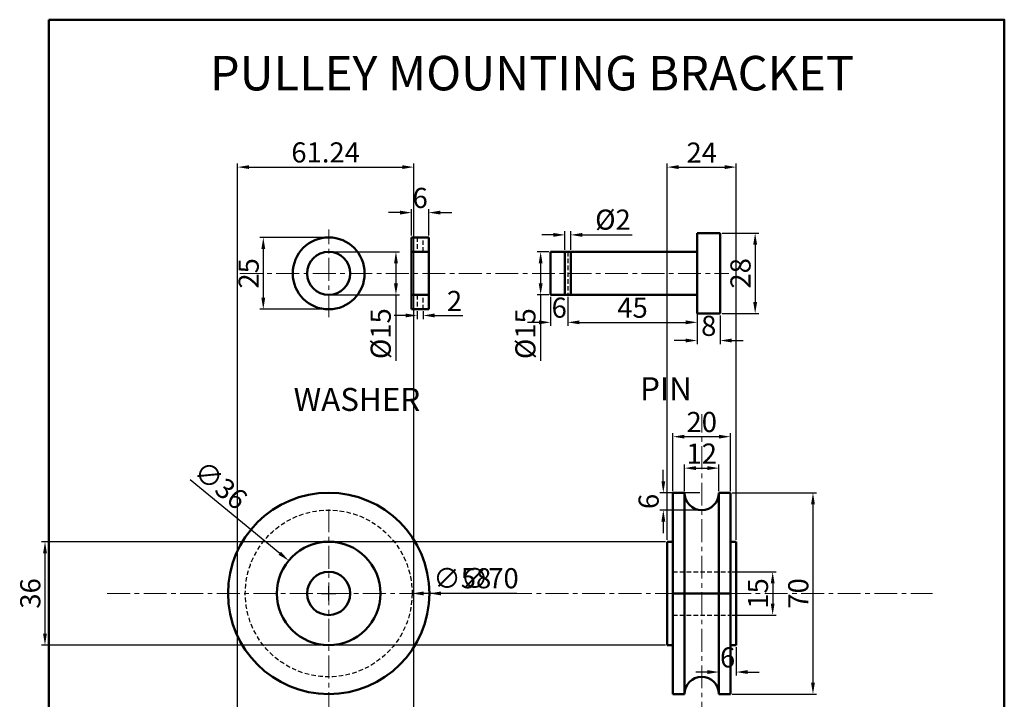
# Model space of a CAD drawing. Units: millimetres. Extents: x 50 to 393, y 3 to 474.
# Tile 2 of 2: x 50 to 393, y 238 to 474. Entities that reach past the tile are written whole.
import ezdxf

# ---------------------------------------------------------------- set-up
doc = ezdxf.new("R2010")
doc.units = ezdxf.units.MM
doc.header["$LTSCALE"] = 0.5
doc.linetypes.add('CENTER', pattern=[50.8, 31.75, -6.35, 6.35, -6.35])
doc.linetypes.add('HIDDEN', pattern=[9.525, 6.35, -3.175])
for name, color, linetype, lineweight in [('M-CNTR', 4, 'CENTER', 18), ('M-DIMS', 2, 'Continuous', 25), ('M-HIDN', 1, 'HIDDEN', 25), ('M-OUTL', 7, 'Continuous', 50), ('M-TEXT', 7, 'Continuous', 25), ('M-TTLB', 7, 'Continuous', 50)]:
    doc.layers.add(name, color=color, linetype=linetype, lineweight=lineweight)
doc.styles.get("Standard").update_dxf_attribs({"font": 'arial.ttf'})
doc.dimstyles.new('ISO-25', dxfattribs={"dimtxt": 7, "dimasz": 4, "dimexe": 1.25, "dimexo": 0.625, "dimtad": 1, "dimtxsty": 'Standard', "dimcen": 2.5, "dimadec": 0, "dimazin": 0, "dimtfac": 1, "dimtofl": 0, "dimtmove": 0, "dimatfit": 3, "dimfxl": 1, "dimarcsym": 0})

# ---------------------------------------------------------------- blocks, each defined once
blk = doc.blocks.new('*D20')
at = {"layer": 'Defpoints', "color": 0, "ltscale": 0.5, "transparency": 16777216}
for p in [(293.48, 318.29), (281.48, 309.71), (293.48, 309.71)]:
    blk.add_point(p, dxfattribs=at)
at = {"layer": 'M-DIMS', "color": 0, "lineweight": -2, "ltscale": 0.5, "transparency": 16777216}
for p, q in [((281.48, 310.33), (281.48, 319.54)), ((293.48, 310.33), (293.48, 319.54)), ((285.48, 318.29), (289.48, 318.29))]:
    blk.add_line(p, q, dxfattribs=at)
at = {"layer": 'M-DIMS', "color": 0, "ltscale": 0.5, "transparency": 16777216}
for points in [[(285.48, 318.96), (285.48, 317.63), (281.48, 318.29)], [(289.48, 318.96), (289.48, 317.63), (293.48, 318.29)]]:
    blk.add_solid(points, dxfattribs=at)
at = {"layer": 'M-DIMS', "color": 0, "ltscale": 0.5, "transparency": 16777216, "insert": (287.48, 322.43), "char_height": 7, "attachment_point": 5}
blk.add_mtext('12', dxfattribs=at)
blk = doc.blocks.new('*D21')
at = {"layer": 'Defpoints', "color": 0, "ltscale": 0.5, "transparency": 16777216}
for p in [(297.48, 282.21), (297.48, 267.21), (312.15, 267.21)]:
    blk.add_point(p, dxfattribs=at)
at = {"layer": 'M-DIMS', "color": 0, "lineweight": -2, "ltscale": 0.5, "transparency": 16777216}
for p, q in [((298.11, 282.21), (313.4, 282.21)), ((312.15, 278.21), (312.15, 271.21)), ((298.11, 267.21), (313.4, 267.21))]:
    blk.add_line(p, q, dxfattribs=at)
at = {"layer": 'M-DIMS', "color": 0, "ltscale": 0.5, "transparency": 16777216}
for points in [[(311.49, 278.21), (312.82, 278.21), (312.15, 282.21)], [(311.49, 271.21), (312.82, 271.21), (312.15, 267.21)]]:
    blk.add_solid(points, dxfattribs=at)
at = {"layer": 'M-DIMS', "color": 0, "ltscale": 0.5, "transparency": 16777216, "insert": (307.95, 274.71), "char_height": 7, "attachment_point": 5, "rotation": 90}
blk.add_mtext('15', dxfattribs=at)
blk = doc.blocks.new('*D22')
at = {"layer": 'Defpoints', "color": 0, "ltscale": 0.5, "transparency": 16777216}
for p in [(297.48, 309.71), (297.48, 239.71), (326.16, 239.71)]:
    blk.add_point(p, dxfattribs=at)
at = {"layer": 'M-DIMS', "color": 0, "lineweight": -2, "ltscale": 0.5, "transparency": 16777216}
for p, q in [((298.11, 309.71), (327.41, 309.71)), ((326.16, 305.71), (326.16, 243.71)), ((298.11, 239.71), (327.41, 239.71))]:
    blk.add_line(p, q, dxfattribs=at)
at = {"layer": 'M-DIMS', "color": 0, "ltscale": 0.5, "transparency": 16777216}
for points in [[(325.49, 305.71), (326.83, 305.71), (326.16, 309.71)], [(325.49, 243.71), (326.83, 243.71), (326.16, 239.71)]]:
    blk.add_solid(points, dxfattribs=at)
at = {"layer": 'M-DIMS', "color": 0, "ltscale": 0.5, "transparency": 16777216, "insert": (321.96, 274.71), "char_height": 7, "attachment_point": 5, "rotation": 90}
blk.add_mtext('70', dxfattribs=at)
blk = doc.blocks.new('*D23')
at = {"layer": 'Defpoints', "color": 0, "ltscale": 0.5, "transparency": 16777216}
for p in [(293.48, 256.71), (299.48, 256.71), (299.48, 247.38)]:
    blk.add_point(p, dxfattribs=at)
at = {"layer": 'M-DIMS', "color": 0, "lineweight": -2, "ltscale": 0.5, "transparency": 16777216}
for p, q in [((293.48, 256.08), (293.48, 246.13)), ((299.48, 256.08), (299.48, 246.13)), ((289.48, 247.38), (285.48, 247.38)), ((303.48, 247.38), (307.48, 247.38))]:
    blk.add_line(p, q, dxfattribs=at)
at = {"layer": 'M-DIMS', "color": 0, "ltscale": 0.5, "transparency": 16777216}
for points in [[(289.48, 248.05), (289.48, 246.71), (293.48, 247.38)], [(303.48, 248.05), (303.48, 246.71), (299.48, 247.38)]]:
    blk.add_solid(points, dxfattribs=at)
at = {"layer": 'M-DIMS', "color": 0, "ltscale": 0.5, "transparency": 16777216, "insert": (296.48, 251.58), "char_height": 7, "attachment_point": 5}
blk.add_mtext('6', dxfattribs=at)
blk = doc.blocks.new('*D24')
at = {"layer": 'Defpoints', "color": 0, "ltscale": 0.5, "transparency": 16777216}
for p in [(274.13, 309.71), (287.48, 309.71), (287.48, 303.71)]:
    blk.add_point(p, dxfattribs=at)
at = {"layer": 'M-DIMS', "color": 0, "lineweight": -2, "ltscale": 0.5, "transparency": 16777216}
for p, q in [((274.13, 313.71), (274.13, 317.71)), ((286.86, 309.71), (272.88, 309.71)), ((286.86, 303.71), (272.88, 303.71)), ((274.13, 299.71), (274.13, 295.71))]:
    blk.add_line(p, q, dxfattribs=at)
at = {"layer": 'M-DIMS', "color": 0, "ltscale": 0.5, "transparency": 16777216}
for points in [[(273.47, 313.71), (274.8, 313.71), (274.13, 309.71)], [(273.47, 299.71), (274.8, 299.71), (274.13, 303.71)]]:
    blk.add_solid(points, dxfattribs=at)
at = {"layer": 'M-DIMS', "color": 0, "ltscale": 0.5, "transparency": 16777216, "insert": (269.93, 306.71), "char_height": 7, "attachment_point": 5, "rotation": 90}
blk.add_mtext('6', dxfattribs=at)
blk = doc.blocks.new('*D25')
at = {"layer": 'Defpoints', "color": 0, "ltscale": 0.5, "transparency": 16777216}
for p in [(143.88, 286.14), (171.7, 263.28)]:
    blk.add_point(p, dxfattribs=at)
at = {"layer": 'M-DIMS', "color": 0, "lineweight": -2, "ltscale": 0.5, "transparency": 16777216}
for p, q in [((109.57, 314.32), (140.79, 288.67)), ((155.29, 274.71), (160.29, 274.71)), ((157.79, 272.21), (157.79, 277.21))]:
    blk.add_line(p, q, dxfattribs=at)
at = {"layer": 'M-DIMS', "color": 0, "ltscale": 0.5, "transparency": 16777216}
blk.add_solid([(141.21, 289.19), (140.36, 288.16), (143.88, 286.14)], dxfattribs=at)
at = {"layer": 'M-DIMS', "color": 0, "ltscale": 0.5, "transparency": 16777216, "insert": (119.66, 311.72), "char_height": 7, "attachment_point": 5, "rotation": 320.6}
blk.add_mtext('∅36', dxfattribs=at)
blk = doc.blocks.new('*D26')
at = {"layer": 'Defpoints', "color": 0, "ltscale": 0.5, "transparency": 16777216}
for p in [(157.79, 398.51), (135.05, 373.51), (157.79, 373.51)]:
    blk.add_point(p, dxfattribs=at)
at = {"layer": 'M-DIMS', "color": 0, "lineweight": -2, "ltscale": 0.5, "transparency": 16777216}
for p, q in [((157.16, 398.51), (133.8, 398.51)), ((135.05, 394.51), (135.05, 377.51)), ((157.16, 373.51), (133.8, 373.51))]:
    blk.add_line(p, q, dxfattribs=at)
at = {"layer": 'M-DIMS', "color": 0, "ltscale": 0.5, "transparency": 16777216}
for points in [[(134.39, 394.51), (135.72, 394.51), (135.05, 398.51)], [(134.39, 377.51), (135.72, 377.51), (135.05, 373.51)]]:
    blk.add_solid(points, dxfattribs=at)
at = {"layer": 'M-DIMS', "color": 0, "ltscale": 0.5, "transparency": 16777216, "insert": (130.86, 386.01), "char_height": 7, "attachment_point": 5, "rotation": 90}
blk.add_mtext('25', dxfattribs=at)
blk = doc.blocks.new('*D27')
at = {"layer": 'Defpoints', "color": 0, "ltscale": 0.5, "transparency": 16777216}
for p in [(157.79, 393.51), (157.79, 378.51), (181.17, 378.51)]:
    blk.add_point(p, dxfattribs=at)
at = {"layer": 'M-DIMS', "color": 0, "lineweight": -2, "ltscale": 0.5, "transparency": 16777216}
for p, q in [((158.41, 393.51), (182.42, 393.51)), ((181.17, 389.51), (181.17, 382.51)), ((158.41, 378.51), (182.42, 378.51)), ((181.17, 378.51), (181.17, 355.57))]:
    blk.add_line(p, q, dxfattribs=at)
at = {"layer": 'M-DIMS', "color": 0, "ltscale": 0.5, "transparency": 16777216}
for points in [[(180.51, 389.51), (181.84, 389.51), (181.17, 393.51)], [(180.51, 382.51), (181.84, 382.51), (181.17, 378.51)]]:
    blk.add_solid(points, dxfattribs=at)
at = {"layer": 'M-DIMS', "color": 0, "ltscale": 0.5, "transparency": 16777216, "insert": (176.78, 365.04), "char_height": 7, "attachment_point": 5, "rotation": 90}
blk.add_mtext('%%C15', dxfattribs=at)
blk = doc.blocks.new('*D28')
at = {"layer": 'Defpoints', "color": 0, "ltscale": 0.5, "transparency": 16777216}
for p in [(192.59, 407.14), (186.59, 398.51), (192.59, 398.51)]:
    blk.add_point(p, dxfattribs=at)
at = {"layer": 'M-DIMS', "color": 0, "lineweight": -2, "ltscale": 0.5, "transparency": 16777216}
for p, q in [((186.59, 399.14), (186.59, 408.39)), ((192.59, 399.14), (192.59, 408.39)), ((182.59, 407.14), (178.59, 407.14)), ((196.59, 407.14), (200.59, 407.14))]:
    blk.add_line(p, q, dxfattribs=at)
at = {"layer": 'M-DIMS', "color": 0, "ltscale": 0.5, "transparency": 16777216}
for points in [[(182.59, 407.81), (182.59, 406.47), (186.59, 407.14)], [(196.59, 407.81), (196.59, 406.47), (192.59, 407.14)]]:
    blk.add_solid(points, dxfattribs=at)
at = {"layer": 'M-DIMS', "color": 0, "ltscale": 0.5, "transparency": 16777216, "insert": (189.59, 411.34), "char_height": 7, "attachment_point": 5}
blk.add_mtext('6', dxfattribs=at)
blk = doc.blocks.new('*D29')
at = {"layer": 'Defpoints', "color": 0, "ltscale": 0.5, "transparency": 16777216}
for p in [(188.59, 373.51), (190.59, 373.51), (190.59, 371.37)]:
    blk.add_point(p, dxfattribs=at)
at = {"layer": 'M-DIMS', "color": 0, "lineweight": -2, "ltscale": 0.5, "transparency": 16777216}
for p, q in [((184.59, 371.37), (180.59, 371.37)), ((188.59, 372.89), (188.59, 370.12)), ((190.59, 372.89), (190.59, 370.12)), ((194.59, 371.37), (204.48, 371.37))]:
    blk.add_line(p, q, dxfattribs=at)
at = {"layer": 'M-DIMS', "color": 0, "ltscale": 0.5, "transparency": 16777216}
for points in [[(184.59, 372.04), (184.59, 370.71), (188.59, 371.37)], [(194.59, 372.04), (194.59, 370.71), (190.59, 371.37)]]:
    blk.add_solid(points, dxfattribs=at)
at = {"layer": 'M-DIMS', "color": 0, "ltscale": 0.5, "transparency": 16777216, "insert": (201.54, 375.51), "char_height": 7, "attachment_point": 5}
blk.add_mtext('2', dxfattribs=at)
blk = doc.blocks.new('*D30')
at = {"layer": 'Defpoints', "color": 0, "ltscale": 0.5, "transparency": 16777216}
for p in [(234.93, 393.51), (231.48, 378.51), (234.93, 378.51)]:
    blk.add_point(p, dxfattribs=at)
at = {"layer": 'M-DIMS', "color": 0, "lineweight": -2, "ltscale": 0.5, "transparency": 16777216}
for p, q in [((234.31, 393.51), (230.23, 393.51)), ((231.48, 389.51), (231.48, 382.51)), ((234.31, 378.51), (230.23, 378.51)), ((231.48, 378.51), (231.48, 355.57))]:
    blk.add_line(p, q, dxfattribs=at)
at = {"layer": 'M-DIMS', "color": 0, "ltscale": 0.5, "transparency": 16777216}
for points in [[(230.81, 389.51), (232.15, 389.51), (231.48, 393.51)], [(230.81, 382.51), (232.15, 382.51), (231.48, 378.51)]]:
    blk.add_solid(points, dxfattribs=at)
at = {"layer": 'M-DIMS', "color": 0, "ltscale": 0.5, "transparency": 16777216, "insert": (227.09, 365.04), "char_height": 7, "attachment_point": 5, "rotation": 90}
blk.add_mtext('%%C15', dxfattribs=at)
blk = doc.blocks.new('*D31')
at = {"layer": 'Defpoints', "color": 0, "ltscale": 0.5, "transparency": 16777216}
for p in [(234.93, 378.51), (240.93, 378.51), (240.93, 368.98)]:
    blk.add_point(p, dxfattribs=at)
at = {"layer": 'M-DIMS', "color": 0, "lineweight": -2, "ltscale": 0.5, "transparency": 16777216}
for p, q in [((234.93, 377.89), (234.93, 367.73)), ((240.93, 377.89), (240.93, 367.73)), ((230.93, 368.98), (226.93, 368.98)), ((244.93, 368.98), (248.93, 368.98))]:
    blk.add_line(p, q, dxfattribs=at)
at = {"layer": 'M-DIMS', "color": 0, "ltscale": 0.5, "transparency": 16777216}
for points in [[(230.93, 369.65), (230.93, 368.32), (234.93, 368.98)], [(244.93, 369.65), (244.93, 368.32), (240.93, 368.98)]]:
    blk.add_solid(points, dxfattribs=at)
at = {"layer": 'M-DIMS', "color": 0, "ltscale": 0.5, "transparency": 16777216, "insert": (237.93, 373.18), "char_height": 7, "attachment_point": 5}
blk.add_mtext('6', dxfattribs=at)
blk = doc.blocks.new('*D32')
at = {"layer": 'Defpoints', "color": 0, "ltscale": 0.5, "transparency": 16777216}
for p in [(241.93, 399.39), (239.93, 393.51), (241.93, 393.51)]:
    blk.add_point(p, dxfattribs=at)
at = {"layer": 'M-DIMS', "color": 0, "lineweight": -2, "ltscale": 0.5, "transparency": 16777216}
for p, q in [((239.93, 394.14), (239.93, 400.64)), ((241.93, 394.14), (241.93, 400.64)), ((235.93, 399.39), (231.93, 399.39)), ((245.93, 399.39), (263.32, 399.39))]:
    blk.add_line(p, q, dxfattribs=at)
at = {"layer": 'M-DIMS', "color": 0, "ltscale": 0.5, "transparency": 16777216}
for points in [[(235.93, 400.06), (235.93, 398.73), (239.93, 399.39)], [(245.93, 400.06), (245.93, 398.73), (241.93, 399.39)]]:
    blk.add_solid(points, dxfattribs=at)
at = {"layer": 'M-DIMS', "color": 0, "ltscale": 0.5, "transparency": 16777216, "insert": (256.62, 403.79), "char_height": 7, "attachment_point": 5}
blk.add_mtext('%%C2', dxfattribs=at)
blk = doc.blocks.new('*D33')
at = {"layer": 'Defpoints', "color": 0, "ltscale": 0.5, "transparency": 16777216}
for p in [(240.93, 375.44), (285.93, 375.44), (285.93, 368.98)]:
    blk.add_point(p, dxfattribs=at)
at = {"layer": 'M-DIMS', "color": 0, "lineweight": -2, "ltscale": 0.5, "transparency": 16777216}
for p, q in [((240.93, 374.81), (240.93, 367.73)), ((285.93, 374.81), (285.93, 367.73)), ((244.93, 368.98), (281.93, 368.98))]:
    blk.add_line(p, q, dxfattribs=at)
at = {"layer": 'M-DIMS', "color": 0, "ltscale": 0.5, "transparency": 16777216}
for points in [[(244.93, 369.65), (244.93, 368.32), (240.93, 368.98)], [(281.93, 369.65), (281.93, 368.32), (285.93, 368.98)]]:
    blk.add_solid(points, dxfattribs=at)
at = {"layer": 'M-DIMS', "color": 0, "ltscale": 0.5, "transparency": 16777216, "insert": (263.43, 373.17), "char_height": 7, "attachment_point": 5}
blk.add_mtext('45', dxfattribs=at)
blk = doc.blocks.new('*D34')
at = {"layer": 'Defpoints', "color": 0, "ltscale": 0.5, "transparency": 16777216}
for p in [(285.93, 371.27), (293.93, 372.01), (293.93, 362.66)]:
    blk.add_point(p, dxfattribs=at)
at = {"layer": 'M-DIMS', "color": 0, "lineweight": -2, "ltscale": 0.5, "transparency": 16777216}
for p, q in [((285.93, 370.65), (285.93, 361.41)), ((293.93, 371.39), (293.93, 361.41)), ((281.93, 362.66), (277.93, 362.66)), ((297.93, 362.66), (301.93, 362.66))]:
    blk.add_line(p, q, dxfattribs=at)
at = {"layer": 'M-DIMS', "color": 0, "ltscale": 0.5, "transparency": 16777216}
for points in [[(281.93, 363.33), (281.93, 361.99), (285.93, 362.66)], [(297.93, 363.33), (297.93, 361.99), (293.93, 362.66)]]:
    blk.add_solid(points, dxfattribs=at)
at = {"layer": 'M-DIMS', "color": 0, "ltscale": 0.5, "transparency": 16777216, "insert": (289.93, 366.86), "char_height": 7, "attachment_point": 5}
blk.add_mtext('8', dxfattribs=at)
blk = doc.blocks.new('*D35')
at = {"layer": 'Defpoints', "color": 0, "ltscale": 0.5, "transparency": 16777216}
for p in [(293.93, 400.01), (293.93, 372.01), (306.06, 372.01)]:
    blk.add_point(p, dxfattribs=at)
at = {"layer": 'M-DIMS', "color": 0, "lineweight": -2, "ltscale": 0.5, "transparency": 16777216}
for p, q in [((294.56, 400.01), (307.31, 400.01)), ((306.06, 396.01), (306.06, 376.01)), ((294.56, 372.01), (307.31, 372.01))]:
    blk.add_line(p, q, dxfattribs=at)
at = {"layer": 'M-DIMS', "color": 0, "ltscale": 0.5, "transparency": 16777216}
for points in [[(305.4, 396.01), (306.73, 396.01), (306.06, 400.01)], [(305.4, 376.01), (306.73, 376.01), (306.06, 372.01)]]:
    blk.add_solid(points, dxfattribs=at)
at = {"layer": 'M-DIMS', "color": 0, "ltscale": 0.5, "transparency": 16777216, "insert": (301.87, 386.01), "char_height": 7, "attachment_point": 5, "rotation": 90}
blk.add_mtext('28', dxfattribs=at)
blk = doc.blocks.new('*D37')
at = {"layer": 'Defpoints', "color": 0, "ltscale": 0.5, "transparency": 16777216}
for p in [(297.48, 329.23), (277.48, 309.71), (297.48, 309.71)]:
    blk.add_point(p, dxfattribs=at)
at = {"layer": 'M-DIMS', "color": 0, "lineweight": -2, "ltscale": 0.5, "transparency": 16777216}
for p, q in [((277.48, 310.33), (277.48, 330.48)), ((281.48, 329.23), (293.48, 329.23)), ((297.48, 310.33), (297.48, 330.48))]:
    blk.add_line(p, q, dxfattribs=at)
at = {"layer": 'M-DIMS', "color": 0, "ltscale": 0.5, "transparency": 16777216}
for points in [[(281.48, 329.89), (281.48, 328.56), (277.48, 329.23)], [(293.48, 329.89), (293.48, 328.56), (297.48, 329.23)]]:
    blk.add_solid(points, dxfattribs=at)
at = {"layer": 'M-DIMS', "color": 0, "ltscale": 0.5, "transparency": 16777216, "insert": (287.48, 333.42), "char_height": 7, "attachment_point": 5}
blk.add_mtext('20', dxfattribs=at)
blk = doc.blocks.new('*D38')
at = {"layer": 'Defpoints', "color": 0, "ltscale": 0.5, "transparency": 16777216}
for p in [(275.48, 292.71), (59.15, 256.71), (275.48, 256.71)]:
    blk.add_point(p, dxfattribs=at)
at = {"layer": 'M-DIMS', "color": 0, "lineweight": -2, "ltscale": 0.5, "transparency": 16777216}
for p, q in [((274.86, 292.71), (57.9, 292.71)), ((59.15, 288.71), (59.15, 260.71)), ((274.86, 256.71), (57.9, 256.71))]:
    blk.add_line(p, q, dxfattribs=at)
at = {"layer": 'M-DIMS', "color": 0, "ltscale": 0.5, "transparency": 16777216}
for points in [[(58.49, 288.71), (59.82, 288.71), (59.15, 292.71)], [(58.49, 260.71), (59.82, 260.71), (59.15, 256.71)]]:
    blk.add_solid(points, dxfattribs=at)
at = {"layer": 'M-DIMS', "color": 0, "ltscale": 0.5, "transparency": 16777216, "insert": (54.95, 274.71), "char_height": 7, "attachment_point": 5, "rotation": 90}
blk.add_mtext('36', dxfattribs=at)
blk = doc.blocks.new('*D39')
at = {"layer": 'Defpoints', "color": 0, "ltscale": 0.5, "transparency": 16777216}
for p in [(299.48, 422.96), (275.48, 292.71), (299.48, 292.71)]:
    blk.add_point(p, dxfattribs=at)
at = {"layer": 'M-DIMS', "color": 0, "lineweight": -2, "ltscale": 0.5, "transparency": 16777216}
for p, q in [((275.48, 293.33), (275.48, 424.21)), ((279.48, 422.96), (295.48, 422.96)), ((299.48, 293.33), (299.48, 424.21))]:
    blk.add_line(p, q, dxfattribs=at)
at = {"layer": 'M-DIMS', "color": 0, "ltscale": 0.5, "transparency": 16777216}
for points in [[(279.48, 423.63), (279.48, 422.29), (275.48, 422.96)], [(295.48, 423.63), (295.48, 422.29), (299.48, 422.96)]]:
    blk.add_solid(points, dxfattribs=at)
at = {"layer": 'M-DIMS', "color": 0, "ltscale": 0.5, "transparency": 16777216, "insert": (287.48, 427.1), "char_height": 7, "attachment_point": 5}
blk.add_mtext('24', dxfattribs=at)
blk = doc.blocks.new('*D40')
at = {"layer": 'Defpoints', "color": 0, "ltscale": 0.5, "transparency": 16777216}
for p in [(187.35, 422.96), (126.11, 165.84), (187.35, 165.94)]:
    blk.add_point(p, dxfattribs=at)
at = {"layer": 'M-DIMS', "color": 0, "lineweight": -2, "ltscale": 0.5, "transparency": 16777216}
for p, q in [((126.11, 166.46), (126.11, 424.21)), ((130.11, 422.96), (183.35, 422.96)), ((187.35, 166.56), (187.35, 424.21))]:
    blk.add_line(p, q, dxfattribs=at)
at = {"layer": 'M-DIMS', "color": 0, "ltscale": 0.5, "transparency": 16777216}
for points in [[(130.11, 423.63), (130.11, 422.29), (126.11, 422.96)], [(183.35, 423.63), (183.35, 422.29), (187.35, 422.96)]]:
    blk.add_solid(points, dxfattribs=at)
at = {"layer": 'M-DIMS', "color": 0, "ltscale": 0.5, "transparency": 16777216, "insert": (156.73, 427.16), "char_height": 7, "attachment_point": 5}
blk.add_mtext('61.24', dxfattribs=at)
blk = doc.blocks.new('*D43')
at = {"layer": 'Defpoints', "color": 0, "ltscale": 0.5, "transparency": 16777216}
for p in [(122.79, 274.71), (192.79, 274.71)]:
    blk.add_point(p, dxfattribs=at)
at = {"layer": 'M-DIMS', "color": 0, "lineweight": -2, "ltscale": 0.5, "transparency": 16777216}
for p, q in [((155.29, 274.71), (160.29, 274.71)), ((157.79, 272.21), (157.79, 277.21)), ((223.22, 274.71), (196.79, 274.71))]:
    blk.add_line(p, q, dxfattribs=at)
at = {"layer": 'M-DIMS', "color": 0, "ltscale": 0.5, "transparency": 16777216}
blk.add_solid([(196.79, 275.38), (196.79, 274.04), (192.79, 274.71)], dxfattribs=at)
at = {"layer": 'M-DIMS', "color": 0, "ltscale": 0.5, "transparency": 16777216, "insert": (213.79, 279.1), "char_height": 7, "attachment_point": 5, "rotation": 0}
blk.add_mtext('∅70', dxfattribs=at)
blk = doc.blocks.new('*D44')
at = {"layer": 'Defpoints', "color": 0, "ltscale": 0.5, "transparency": 16777216}
for p in [(128.79, 274.71), (186.79, 274.71)]:
    blk.add_point(p, dxfattribs=at)
at = {"layer": 'M-DIMS', "color": 0, "lineweight": -2, "ltscale": 0.5, "transparency": 16777216}
for p, q in [((155.29, 274.71), (160.29, 274.71)), ((157.79, 272.21), (157.79, 277.21)), ((213.69, 274.71), (190.79, 274.71))]:
    blk.add_line(p, q, dxfattribs=at)
at = {"layer": 'M-DIMS', "color": 0, "ltscale": 0.5, "transparency": 16777216}
blk.add_solid([(190.79, 275.38), (190.79, 274.04), (186.79, 274.71)], dxfattribs=at)
at = {"layer": 'M-DIMS', "color": 0, "ltscale": 0.5, "transparency": 16777216, "insert": (204.24, 279.1), "char_height": 7, "attachment_point": 5, "rotation": 0}
blk.add_mtext('∅58', dxfattribs=at)

msp = doc.modelspace()

# ---------------------------------------------------------------- linework, layer by layer
at = {"layer": 'M-CNTR', "ltscale": 0.5}
for p, q in [((157.787, 370.733), (157.787, 401.308)), ((126.881, 386.011), (296.957, 386.011)), ((287.481, 63.964), (287.481, 337.045)), ((157.787, 303.93), (157.787, 57.07)), ((80.803, 274.71), (367.747, 274.71))]:
    msp.add_line(p, q, dxfattribs=at)
at = {"layer": 'M-HIDN', "ltscale": 0.5}
for p, q in [((188.592, 398.511), (188.592, 393.511)), ((190.592, 393.511), (190.592, 398.511)), ((240.933, 393.511), (240.933, 378.511)), ((188.592, 378.511), (188.592, 373.511)), ((190.592, 373.511), (190.592, 378.511)), ((277.481, 282.21), (297.481, 282.21)), ((277.481, 267.21), (297.481, 267.21))]:
    msp.add_line(p, q, dxfattribs=at)
msp.add_circle((157.787, 274.71), 29, dxfattribs=at)
at = {"layer": 'M-OUTL', "ltscale": 0.5}
for p, q in [((186.592, 373.511), (186.592, 398.511)), ((186.592, 398.511), (192.592, 398.511)), ((192.592, 398.511), (192.592, 373.511)), ((293.933, 400.011), (285.933, 400.011)), ((285.933, 400.011), (285.933, 372.011)), ((293.933, 386.011), (293.933, 400.011)), ((186.592, 393.511), (192.592, 393.511)), ((285.933, 393.511), (234.933, 393.511)), ((234.933, 393.511), (234.933, 378.511)), ((239.933, 393.511), (239.933, 378.511)), ((241.933, 393.511), (241.933, 378.511)), ((293.933, 372.011), (293.933, 386.011)), ((186.592, 378.511), (192.592, 378.511)), ((234.933, 378.511), (285.933, 378.511)), ((192.592, 373.511), (186.592, 373.511)), ((285.933, 372.011), (293.933, 372.011)), ((277.481, 309.71), (281.481, 309.71)), ((277.481, 239.71), (277.481, 309.71)), ((281.481, 309.71), (281.481, 239.71)), ((297.481, 309.71), (293.481, 309.71)), ((293.481, 309.71), (293.481, 239.71)), ((297.481, 239.71), (297.481, 309.71)), ((277.481, 292.71), (275.481, 292.71)), ((275.481, 292.71), (275.481, 256.71)), ((297.481, 292.71), (299.481, 292.71)), ((299.481, 292.71), (299.481, 256.71)), ((277.481, 274.71), (297.481, 274.71)), ((275.481, 256.71), (277.481, 256.71)), ((299.481, 256.71), (297.481, 256.71)), ((281.481, 239.71), (277.481, 239.71)), ((277.481, 239.71), (281.481, 239.71)), ((293.481, 239.71), (297.481, 239.71))]:
    msp.add_line(p, q, dxfattribs=at)
for centre, radius in [((157.787, 386.011), 12.5), ((157.787, 386.011), 7.5), ((157.787, 274.71), 35), ((157.787, 274.71), 18), ((157.787, 274.71), 7.5)]:
    msp.add_circle(centre, radius, dxfattribs=at)
for centre, start, end in [((287.481, 309.71), 180, 0), ((287.481, 239.71), 0, 180)]:
    msp.add_arc(centre, 6, start, end, dxfattribs=at)
at = {"layer": 'M-TTLB', "ltscale": 0.5}
msp.add_lwpolyline([(60.52, 474.222), (392.686, 474.222), (392.686, 3.466), (60.52, 3.466)], close=True, dxfattribs=at)

# ---------------------------------------------------------------- texts
at = {"layer": 'M-TEXT', "ltscale": 0.5, "attachment_point": 1}
for s, width, insert, char_height in [('\\pxqc;PULLEY MOUNTING BRACKET', 231.58139, (112.657, 461.639), 12), ('\\pxqc;PIN', 45.18848, (252.447, 349.906), 8), ('WASHER', 45.18848, (145.599, 346.174), 8)]:
    msp.add_mtext_dynamic_manual_height_columns(s, width=width, gutter_width=12.5, heights=[0], dxfattribs=dict(at, insert=insert, char_height=char_height))

# ---------------------------------------------------------------- dimensions: what is measured, and where the dimension line sits
at = {"layer": 'M-DIMS', "ltscale": 0.5}
for base, p1, p2, override, picture, middle in [((187.346, 422.958), (126.108, 165.835), (187.346, 165.937), {"dimdec": 2, "dimlfac": 1, "dimrnd": 0, "dimzin": 0, "dimdsep": 46, "dimlunit": 2}, '*D40', (156.727, 427.157)), ((299.481, 422.958), (275.481, 292.71), (299.481, 292.71), {"dimdec": 0, "dimlfac": 1, "dimrnd": 0, "dimzin": 0, "dimdsep": 46, "dimlunit": 2}, '*D39', (287.481, 427.098)), ((192.592, 407.14), (186.592, 398.511), (192.592, 398.511), {"dimclrd": 0, "dimclre": 0, "dimclrt": 0}, '*D28', (189.592, 411.339)), ((190.592, 371.373), (188.592, 373.511), (190.592, 373.511), {"dimclrd": 0, "dimclre": 0, "dimclrt": 0}, '*D29', (201.535, 375.512)), ((240.933, 368.984), (234.933, 378.511), (240.933, 378.511), {"dimclrd": 0, "dimclre": 0, "dimclrt": 0}, '*D31', (237.933, 373.183)), ((285.933, 368.984), (240.933, 375.439), (285.933, 375.439), {"dimclrd": 0, "dimclre": 0, "dimclrt": 0}, '*D33', (263.433, 373.169)), ((293.933, 362.661), (285.933, 371.274), (293.933, 372.011), {"dimclrd": 0, "dimclre": 0, "dimclrt": 0}, '*D34', (289.933, 366.86)), ((297.481, 329.225), (277.481, 309.71), (297.481, 309.71), {"dimclrd": 0, "dimclre": 0, "dimclrt": 0}, '*D37', (287.481, 333.424)), ((293.481, 318.295), (281.481, 309.71), (293.481, 309.71), {"dimclrd": 0, "dimclre": 0, "dimclrt": 0}, '*D20', (287.481, 322.434)), ((299.481, 247.381), (293.481, 256.71), (299.481, 256.71), {"dimclrd": 0, "dimclre": 0, "dimclrt": 0}, '*D23', (296.481, 251.58))]:
    dim = msp.add_linear_dim(base=base, p1=p1, p2=p2, dimstyle='ISO-25', override=override, dxfattribs=at)
    dim.commit()
    dim.dimension.update_dxf_attribs({"geometry": picture, "text_midpoint": middle})
dim = msp.add_linear_dim(base=(241.933, 399.394), p1=(239.933, 393.511), p2=(241.933, 393.511), text='%%C<>', dimstyle='ISO-25', override={"dimclrd": 0, "dimclre": 0, "dimclrt": 0}, dxfattribs=at)
dim.commit()
dim.dimension.update_dxf_attribs({"geometry": '*D32', "text_midpoint": (256.625, 403.789)})
for base, p1, p2, override, picture, middle in [((135.054, 373.511), (157.787, 398.511), (157.787, 373.511), {"dimclrd": 0, "dimclre": 0, "dimclrt": 0}, '*D26', (130.855, 386.011)), ((306.065, 372.011), (293.933, 400.011), (293.933, 372.011), {"dimclrd": 0, "dimclre": 0, "dimclrt": 0}, '*D35', (301.866, 386.011)), ((274.132, 309.71), (287.481, 303.71), (287.481, 309.71), {"dimclrd": 0, "dimclre": 0, "dimclrt": 0}, '*D24', (269.933, 306.71)), ((326.16, 239.71), (297.481, 309.71), (297.481, 239.71), {"dimclrd": 0, "dimclre": 0, "dimclrt": 0}, '*D22', (321.961, 274.71)), ((59.153, 256.71), (275.481, 292.71), (275.481, 256.71), {"dimdec": 0, "dimlfac": 1, "dimrnd": 0, "dimzin": 0, "dimdsep": 46, "dimlunit": 2}, '*D38', (54.951, 274.71)), ((312.154, 267.21), (297.481, 282.21), (297.481, 267.21), {"dimclrd": 0, "dimclre": 0, "dimclrt": 0}, '*D21', (307.955, 274.71))]:
    dim = msp.add_linear_dim(base=base, p1=p1, p2=p2, angle=90, dimstyle='ISO-25', override=override, dxfattribs=at)
    dim.commit()
    dim.dimension.update_dxf_attribs({"geometry": picture, "text_midpoint": middle})
for base, p1, p2, picture, middle in [((181.173, 378.511), (157.787, 393.511), (157.787, 378.511), '*D27', (176.778, 365.038)), ((231.481, 378.511), (234.933, 393.511), (234.933, 378.511), '*D30', (227.086, 365.038))]:
    dim = msp.add_linear_dim(base=base, p1=p1, p2=p2, angle=90, text='%%C<>', dimstyle='ISO-25', override={"dimclrd": 0, "dimclre": 0, "dimclrt": 0}, dxfattribs=at)
    dim.commit()
    dim.dimension.update_dxf_attribs({"geometry": picture, "text_midpoint": middle})
for p1, p2, override, picture, middle in [((171.696, 263.285), (143.877, 286.135), {"dimclrd": 0, "dimclre": 0, "dimclrt": 0}, '*D25', (116.868, 308.321)), ((122.787, 274.71), (192.787, 274.71), {"dimdec": 0, "dimlfac": 1, "dimrnd": 0, "dimzin": 0, "dimdsep": 46, "dimlunit": 2}, '*D43', (213.787, 274.71))]:
    dim = msp.add_diameter_dim_2p(p1=p1, p2=p2, dimstyle='ISO-25', override=override, dxfattribs=at)
    dim.commit()
    dim.dimension.update_dxf_attribs({"geometry": picture, "text_midpoint": middle, "dimtype": 163})
dim = msp.add_diameter_dim_2p(p1=(128.787, 274.71), p2=(186.787, 274.71), dimstyle='ISO-25', override={"dimdec": 0, "dimlfac": 1, "dimrnd": 0, "dimzin": 0, "dimdsep": 46, "dimlunit": 2}, dxfattribs=at)
dim.commit()
dim.dimension.update_dxf_attribs({"geometry": '*D44', "text_midpoint": (204.24, 274.71)})

doc.saveas('drawing.dxf')
